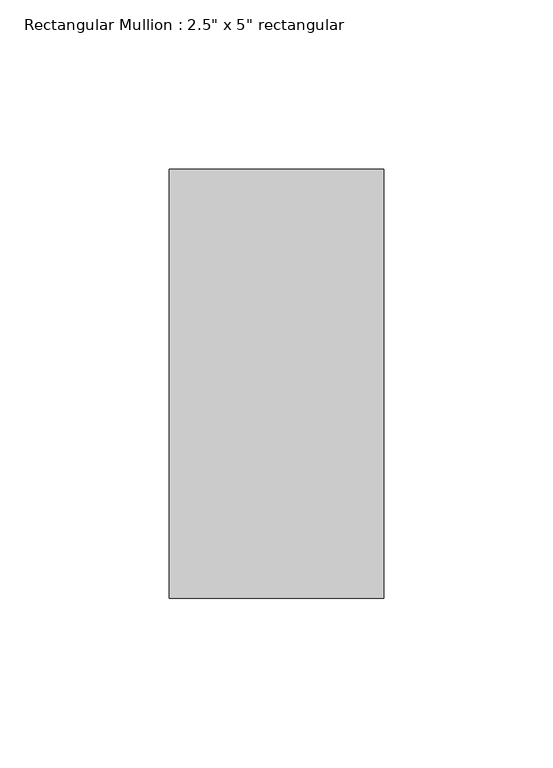
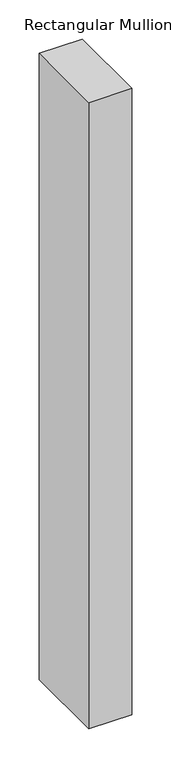
"""IFC4 building model written with IfcOpenShell, lengths in millimetres: member geometry."""

from ifc_helpers import new_model, si_unit, frame, origin, place, context, project, spatial, polyline, outline, extrude, source, transform, mapped, element, save


def member_76e31e9c(model_context):
    return source(origin(), model_context, "Body", "SweptSolid", [
        extrude(outline(polyline([(31.75, 63.5), (31.75, -63.5), (-31.75, -63.5), (-31.75, 63.5), (31.75, 63.5)])), frame((0.0, 0.0, -977.634107), z_axis=(0.0, 0.0, 1.0), x_axis=(1.0, 0.0, 0.0)), (0.0, 0.0, 1.0), 977.634107),
    ])


if __name__ == "__main__":
    model = new_model("IFC4")
    model_context = context("Model", 3, world=origin())
    ifc_project = project(units=[si_unit("LENGTHUNIT", "METRE", prefix="MILLI")], contexts=[model_context])
    site = spatial("IfcSite", under=ifc_project)
    building = spatial("IfcBuilding", under=site)
    placement = place(None, origin())
    member_shape = member_76e31e9c(model_context)
    element("IfcMember", 1, ObjectType="Rectangular Mullion : 2.5\" x 5\" rectangular", at=placement, inside=building, context=model_context, shape_type="MappedRepresentation", body=[
        mapped(member_shape, transform((0.0, 0.0, 0.0), x_axis=(1.0, 0.0, 0.0), y_axis=(0.0, 1.0, 0.0), z_axis=(0.0, 0.0, 1.0))),
    ])
    save(model, "model.ifc")

# Revit data of these elements
# Type "Rectangular Mullion : 2.5\" x 5\" rectangular"
#   built-in parameter 1007304 = 0.416667 (stored number, unit not read)
#   built-in parameter 1007301 = 0.104167 (stored number, unit not read)
#   built-in parameter 1007300 = 0.104167 (stored number, unit not read)
# Element 1 (IfcMember, "Rectangular Mullion : 2.5\" x 5\" rectangular")
#   Materials on its faces: "Roofing, EPDM Membrane"
# Materials
#   "Roofing, EPDM Membrane": class "Generic", colour RGB 127 127 127, transparency 0, Description = "EPDM roof membrane", Cost = 0
